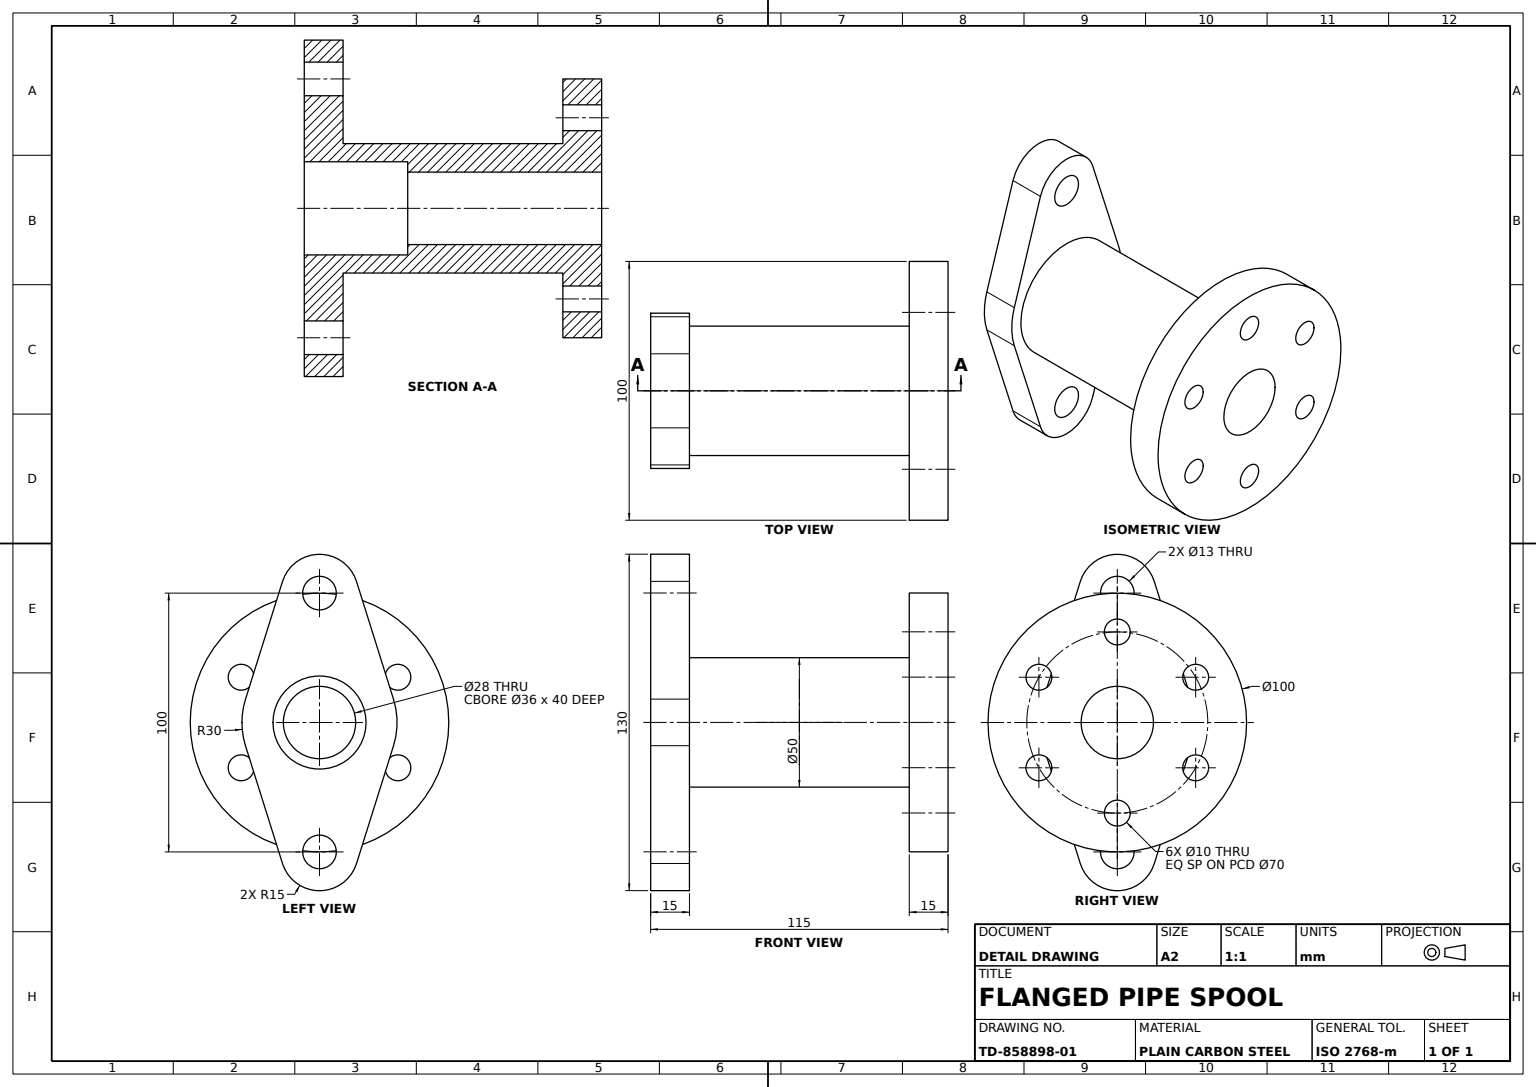
SolidWorks part; units mm, degrees
material "Plain Carbon Steel"
ref_plane "Front Plane" through (0, 0, 0) normal (0, 0, 1) x (1, 0, 0)
ref_plane "Top Plane" through (0, 0, 0) normal (0, 1, 0) x (1, 0, 0)
ref_plane "Right Plane" through (0, 0, 0) normal (1, 0, 0) x (0, 0, -1)
sketch "Round Flange Sketch" plane through (0, 0, 0) normal (0, 0, 1) x (1, 0, 0)
  circle A0 centre (0, 0) radius 50
  dimension "D1" = 100
extrude "Round Flange Ø100" add sketch "Round Flange Sketch" along normal blind 15
sketch "Round Flange Bolt Holes Sketch" plane through (0, 0, 15) normal (0, 0, 1) x (1, 0, 0)
  line L0 (0, 0) -> (0.0794, 0)
  line L1 (0.0794, 0) -> (0, 0)
  line L5 (0, 0) -> (0.0794, 0) construction
  circle A1 centre (0, 35) radius 5
  circle A2 centre (0, -35) radius 5
  circle A3 centre (-30.3109, 17.5) radius 5
  circle A4 centre (-30.3109, -17.5) radius 5
  circle A5 centre (30.3109, -17.5) radius 5
  circle A6 centre (30.3109, 17.5) radius 5
  circle A7 centre (0, 0) radius 50 construction
  dimension "D1" = 10
  dimension "D3" = 10
  dimension "D4" = 10
  dimension "D5" = 10
  dimension "D2" = 10
  dimension "D6" = 10
  dimension "D7" = 0.0794
  dimension "D8" = 30.3109
  dimension "D9" = 30.3109
  dimension "D10" = 17.5
  dimension "D11" = 35
  dimension "D12" = 17.5
  dimension "D13" = 35
extrude "Round Flange Bolt Holes" cut sketch "Round Flange Bolt Holes Sketch" against normal blind 15 contours A3 | A1 | A6 | A4 | A5 | A2
sketch "Spool Core Sketch" plane through (0, 0, 15) normal (0, 0, 1) x (1, 0, 0)
  circle A0 centre (0, 0) radius 18
  dimension "D1" = 36
  dimension "D2" = 36
extrude "Spool Core Ø36" add sketch "Spool Core Sketch" along normal blind 85
sketch "Core Bore Sketch" plane through (0, 0, 100) normal (0, 0, 1) x (1, 0, 0)
  circle A0 centre (0, 0) radius 18
  dimension "D1" = 36
  dimension "D2" = 36
extrude "Core Bore Ø36" cut sketch "Core Bore Sketch" against normal blind 85
sketch "Spool Pipe Sketch" plane through (0, 0, 15) normal (0, 0, 1) x (1, 0, 0)
  circle A0 centre (0, 0) radius 25
  dimension "D1" = 50
  dimension "D2" = 50
extrude "Spool Pipe Ø50" add sketch "Spool Pipe Sketch" along normal blind 85
sketch "Oval Flange Sketch" plane through (0, 0, 100) normal (0, 0, 1) x (1, 0, 0)
  line L2 (-28.6182, 9) -> (-14.3091, 54.5)
  line L3 (-28.6182, -9) -> (-14.3091, -54.5)
  line L4 (14.3091, 54.5) -> (28.6182, 9)
  line L5 (14.3091, -54.5) -> (28.6182, -9)
  arc A0 (14.3091, 54.5) -> (-14.3091, 54.5) centre (0, 50) ccw
  circle A1 centre (0, 0) radius 50 construction
  arc A2 (-14.3091, -54.5) -> (14.3091, -54.5) centre (0, -50) ccw
  arc A3 (-28.6182, 9) -> (-28.6182, -9) centre (0, 0) ccw
  arc A4 (28.6182, -9) -> (28.6182, 9) centre (0, 0) ccw
  dimension "D1" = 30
  dimension "D2" = 30
  dimension "D3" = 60
  dimension "D4" = 15
  dimension "D5" = 30
extrude "Oval Flange" add sketch "Oval Flange Sketch" along normal blind 15
sketch "Oval Flange Holes Sketch" plane through (0, 0, 115) normal (0, 0, 1) x (1, 0, 0)
  circle A0 centre (0, 50) radius 6.5
  circle A1 centre (0, -50) radius 6.5
  dimension "D1" = 13
  dimension "D2" = 13
  dimension "D3" = 13
extrude "Oval Flange Holes 2xØ13" cut sketch "Oval Flange Holes Sketch" against normal blind 15
sketch "Oval Flange Bore Sketch" plane through (0, 0, 115) normal (0, 0, 1) x (1, 0, 0)
  circle A0 centre (0, 0) radius 18
  dimension "D1" = 36
  dimension "D2" = 36
extrude "Oval Flange Bore Ø36" cut sketch "Oval Flange Bore Sketch" against normal blind 40
sketch "Through Bore Sketch" plane through (0, 0, 75) normal (0, 0, 1) x (1, 0, 0)
  circle A0 centre (0, 0) radius 14
  dimension "D1" = 28
  dimension "D2" = 28
extrude "Through Bore Ø28" cut sketch "Through Bore Sketch" against normal blind 75
